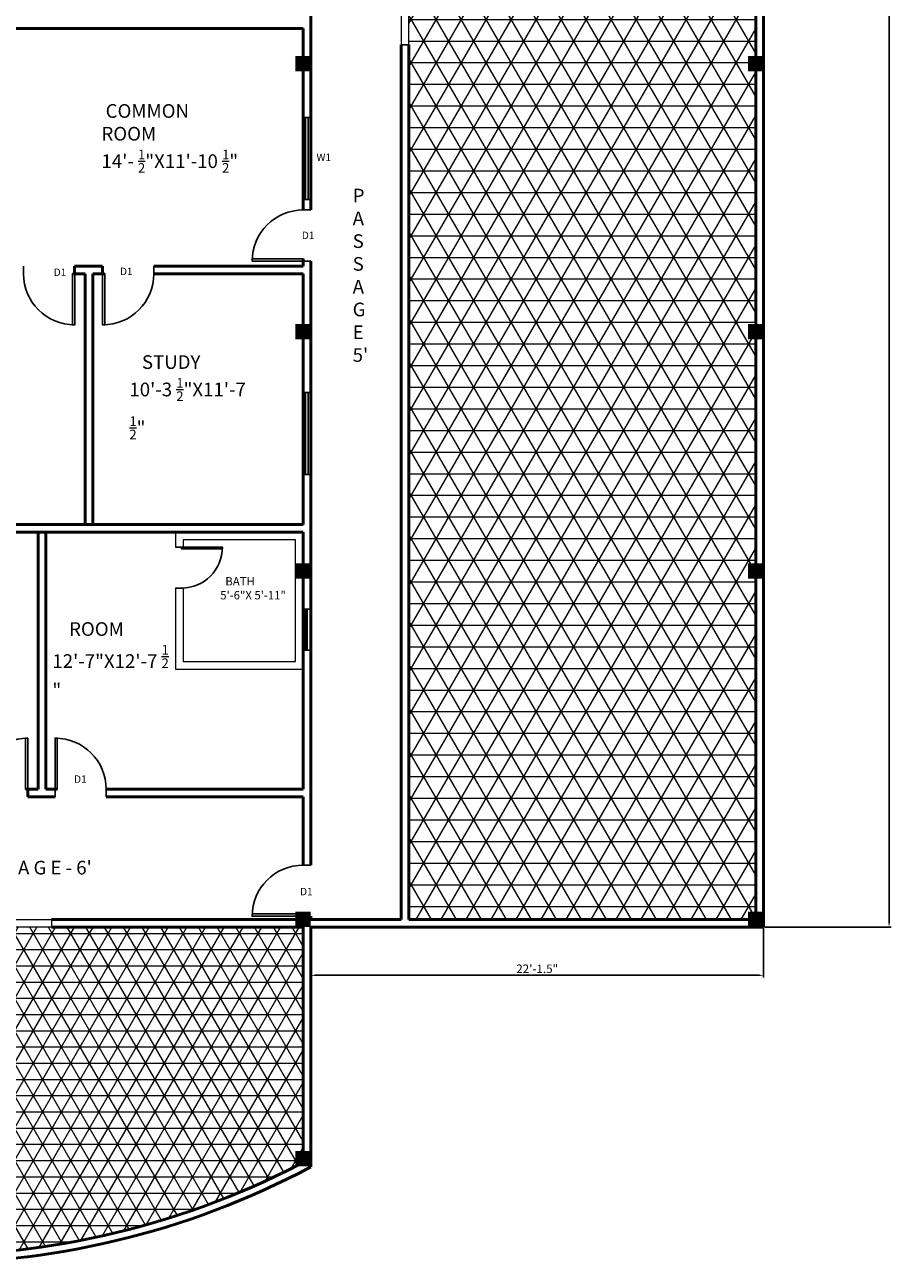
# Model space of a CAD drawing. Units: inches. Extents: x -2733 to 3435, y -338 to 1843.
# Tile 6 of 7: x 1232 to 1741, y 349 to 1076. Entities that reach past the tile are written whole.
import ezdxf

# ---------------------------------------------------------------- set-up
doc = ezdxf.new("R2010")
doc.units = ezdxf.units.IN
doc.header["$PDMODE"] = 34
for name, color, linetype, lineweight in [('A-ANNO-DIMS', 2, 'Continuous', 18), ('A-ANNO-TEXT', 7, 'Continuous', 18), ('A-AREA-IDEN', 3, 'Continuous', 18), ('A-COLS', 1, 'Continuous', 35), ('A-DOOR', 1, 'Continuous', 25), ('A-FLOR-FIXT', 8, 'Continuous', 18), ('A-FLOR-PATT', 9, 'Continuous', 13), ('A-GLAZ', 4, 'Continuous', 25), ('A-WALL', 7, 'Continuous', 50)]:
    doc.layers.add(name, color=color, linetype=linetype, lineweight=lineweight)
doc.styles.get("Standard").update_dxf_attribs({"font": 'arial.ttf'})
doc.styles.add('YQ_DIM', font='SUPEROS.SHX', dxfattribs={"width": 0.8, "bigfont": 'HZDX.SHX'})
doc.dimstyles.new('ISO-25', dxfattribs={"dimtxt": 5, "dimasz": 2.5, "dimexe": 1.25, "dimexo": 0.625, "dimtad": 1, "dimlunit": 3, "dimtxsty": 'Standard', "dimcen": 2.5, "dimadec": 0, "dimazin": 0, "dimtfac": 1, "dimtmove": 0, "dimatfit": 3, "dimfxl": 1, "dimarcsym": 0})

# ---------------------------------------------------------------- blocks, each defined once
blk = doc.blocks.new('*U21')
for p, q in [((0, 0), (0, -6)), ((40, 0), (40, -6))]:
    blk.add_line(p, q)
blk.add_lwpolyline([(0, 0), (0, 40), (1.75, 40), (1.75, 0)], close=True)
blk.add_arc((0, 0), 40, 0, 90)
blk = doc.blocks.new('*D23')
at = {"layer": 'A-ANNO-DIMS', "color": 0, "lineweight": -2, "transparency": 16777216}
for p, q in [((1666.36, 1675.07), (1740.68, 1675.07)), ((1739.43, 1672.57), (1739.43, 549.07)), ((1666.36, 546.57), (1740.68, 546.57))]:
    blk.add_line(p, q, dxfattribs=at)
at = {"layer": 'A-ANNO-DIMS', "color": 0, "lineweight": 20, "transparency": 16777216}
for points in [[(1739.02, 1672.57), (1739.85, 1672.57), (1739.43, 1675.07)], [(1739.02, 549.07), (1739.85, 549.07), (1739.43, 546.57)]]:
    blk.add_solid(points, dxfattribs=at)
at = {"layer": 'Defpoints', "color": 0, "lineweight": 20, "transparency": 16777216}
for p in [(1665.73, 1675.07), (1665.73, 546.57), (1739.43, 546.57)]:
    blk.add_point(p, dxfattribs=at)
at = {"layer": 'A-ANNO-DIMS', "color": 0, "transparency": 16777216, "insert": (1736.26, 1110.82), "char_height": 5, "attachment_point": 5, "rotation": 90}
blk.add_mtext('94\'-0.5"', dxfattribs=at)
blk = doc.blocks.new('*D28')
at = {"layer": 'A-ANNO-DIMS', "color": 0, "lineweight": -2, "ltscale": 0.5, "transparency": 16777216}
for p, q in [((1665.73, 545.95), (1665.73, 517.09)), ((1400.23, 530.41), (1400.23, 517.09)), ((1402.73, 518.34), (1663.23, 518.34))]:
    blk.add_line(p, q, dxfattribs=at)
at = {"layer": 'A-ANNO-DIMS', "color": 0, "lineweight": 20, "ltscale": 0.5, "transparency": 16777216}
for points in [[(1402.73, 518.76), (1402.73, 517.92), (1400.23, 518.34)], [(1663.23, 518.76), (1663.23, 517.92), (1665.73, 518.34)]]:
    blk.add_solid(points, dxfattribs=at)
at = {"layer": 'Defpoints', "color": 0, "lineweight": 20, "ltscale": 0.5, "transparency": 16777216}
for p in [(1665.73, 546.57), (1400.23, 531.04), (1665.73, 518.34)]:
    blk.add_point(p, dxfattribs=at)
at = {"layer": 'A-ANNO-DIMS', "color": 0, "ltscale": 0.5, "transparency": 16777216, "insert": (1532.98, 521.52), "char_height": 5, "attachment_point": 5}
blk.add_mtext('22\'-1.5"', dxfattribs=at)
blk = doc.blocks.new('WIN-1200')
for points in [[(0, 48), (4.5, 48), (4.5, 0), (0, 0)], [(1.29, 48), (2.82, 48), (2.82, 0), (1.29, 0)]]:
    blk.add_lwpolyline(points, close=True)
blk = doc.blocks.new('VENT-600')
at = {"ltscale": 0.5}
for points in [[(0, 24), (4.5, 24), (4.5, 0), (0, 0)], [(1.39, 24), (2.25, 24), (2.25, 0), (1.39, 0)]]:
    blk.add_lwpolyline(points, close=True, dxfattribs=at)

msp = doc.modelspace()

# ---------------------------------------------------------------- hatches: boundary and pattern name
at = {"layer": 'A-COLS'}
h = msp.add_hatch(color=256, dxfattribs=at)
h.dxf.hatch_style = 1
h.paths.add_polyline_path([(1400.159, 1057.953), (1391.159, 1057.953), (1391.159, 1048.953), (1400.159, 1048.953)])
h = msp.add_hatch(color=256, dxfattribs=at)
h.dxf.hatch_style = 1
h.paths.add_polyline_path([(1665.735, 1057.953), (1656.735, 1057.953), (1656.735, 1048.953), (1665.735, 1048.953)])
h = msp.add_hatch(color=256, dxfattribs=at)
h.dxf.hatch_style = 1
h.paths.add_polyline_path([(1400.159, 900.631), (1391.159, 900.631), (1391.159, 891.631), (1400.159, 891.631)])
h = msp.add_hatch(color=256, dxfattribs=at)
h.dxf.hatch_style = 1
h.paths.add_polyline_path([(1665.735, 900.631), (1656.735, 900.631), (1656.735, 891.631), (1665.735, 891.631)])
h = msp.add_hatch(color=256, dxfattribs=at)
h.dxf.hatch_style = 1
h.paths.add_polyline_path([(1400.159, 760.101), (1391.159, 760.101), (1391.159, 751.101), (1400.159, 751.101)])
h = msp.add_hatch(color=256, dxfattribs=at)
h.dxf.hatch_style = 1
h.paths.add_polyline_path([(1665.735, 760.101), (1656.735, 760.101), (1656.735, 751.101), (1665.735, 751.101)])
h = msp.add_hatch(color=256, dxfattribs=at)
h.dxf.hatch_style = 1
h.paths.add_polyline_path([(1400.159, 555.665), (1391.159, 555.665), (1391.159, 546.665), (1400.159, 546.665)])
h = msp.add_hatch(color=256, dxfattribs=at)
h.dxf.hatch_style = 1
h.paths.add_polyline_path([(1665.735, 555.665), (1656.735, 555.665), (1656.735, 546.665), (1665.735, 546.665)])
h = msp.add_hatch(color=256, dxfattribs=at)
h.dxf.hatch_style = 1
h.paths.add_polyline_path([(1400.159, 415.169), (1391.159, 415.169), (1391.159, 406.169), (1400.159, 406.169)])
at = {"layer": 'A-FLOR-PATT'}
h = msp.add_hatch(dxfattribs=at)
h.set_pattern_fill('NET3', color=256, scale=4)
h.paths.add_polyline_path([(1661.235, 1509.072), (1656.735, 1509.072), (1656.735, 1517.29), (1457.735, 1517.29), (1457.735, 1513.572), (1487.735, 1513.572), (1487.735, 1512.26), (1487.706, 1512.26, -0.4014527), (1457.735, 1483.572), (1457.735, 551.072), (1661.235, 551.072)])
h = msp.add_hatch(dxfattribs=at)
h.set_pattern_fill('NET3', color=256, scale=3)
h.paths.add_polyline_path([(1395.735, 546.572), (1089.235, 546.572), (1089.235, 492.572), (964.407, 526.719), (942.472, 413.369, 0.252088), (1395.735, 408.558)])

# ---------------------------------------------------------------- linework, layer by layer
at = {"layer": 'A-FLOR-FIXT', "ltscale": 0.5}
for p, q in [((1453.235, 1214.213), (1453.235, 1064.597)), ((1457.735, 1064.597), (1457.735, 1214.213)), ((1453.235, 1064.597), (1457.735, 1064.597)), ((1176.117, 551.072), (1248.117, 551.072)), ((1248.117, 546.572), (1176.117, 546.572)), ((1248.117, 551.072), (1248.117, 546.572))]:
    msp.add_line(p, q, dxfattribs=at)
at = {"layer": 'A-FLOR-FIXT'}
for p, q in [((1395.735, 967.628), (1400.235, 967.628)), ((1308.059, 934.572), (1308.059, 930.156)), ((1395.735, 937.628), (1400.235, 937.628)), ((1320.735, 769.698), (1325.235, 769.698)), ((1320.735, 745.698), (1325.235, 745.698)), ((1280.124, 627.572), (1280.124, 623.072)), ((1400.235, 583.043), (1395.735, 583.043)), ((1395.735, 553.043), (1400.235, 553.043))]:
    msp.add_line(p, q, dxfattribs=at)
for points in [[(1320.735, 745.698), (1320.735, 698.072), (1395.735, 698.072), (1395.735, 778.572), (1320.735, 778.572), (1320.735, 769.698)], [(1325.235, 745.714), (1325.235, 702.572), (1391.235, 702.572), (1391.235, 774.072), (1325.235, 774.072), (1325.235, 768.648)]]:
    msp.add_lwpolyline(points, dxfattribs=at)
at = {"layer": 'A-GLAZ', "ltscale": 0.5}
msp.add_line((1453.235, 1064.597), (1457.735, 1064.597), dxfattribs=at)
at = {"layer": 'A-WALL'}
for p, q in [((1665.735, 1675.072), (1665.735, 546.572)), ((1661.235, 1509.072), (1661.235, 551.072)), ((1400.235, 1082.676), (1400.235, 967.628)), ((1395.735, 1074.072), (1221.235, 1074.072)), ((1395.735, 1074.072), (1395.735, 967.628)), ((1453.235, 1064.597), (1453.235, 551.072)), ((1457.735, 1064.597), (1457.735, 551.072)), ((1395.735, 938.941), (1395.735, 934.572)), ((1261.606, 934.572), (1261.606, 930.072)), ((1277.992, 934.572), (1261.606, 934.572)), ((1277.992, 934.572), (1277.992, 930.072)), ((1395.735, 934.572), (1308.059, 934.572)), ((1400.235, 937.628), (1400.235, 583.043)), ((1267.735, 930.072), (1260.556, 930.072)), ((1267.735, 930.072), (1267.735, 783.072)), ((1272.235, 930.072), (1272.235, 783.072)), ((1279.042, 930.072), (1272.235, 930.072)), ((1395.735, 930.072), (1308.059, 930.072)), ((1395.735, 930.072), (1395.735, 783.072)), ((1395.735, 783.072), (1018.896, 783.072)), ((1395.735, 778.572), (1089.235, 778.572)), ((1240.235, 778.572), (1240.235, 627.572)), ((1244.735, 778.572), (1244.735, 627.572)), ((1395.735, 778.572), (1395.735, 627.572)), ((1240.235, 627.572), (1233.067, 627.572)), ((1234.117, 627.572), (1234.117, 623.072)), ((1251.437, 627.572), (1244.735, 627.572)), ((1395.735, 627.572), (1280.124, 627.572)), ((1250.124, 623.072), (1234.117, 623.072)), ((1395.735, 623.072), (1280.124, 623.072)), ((1395.735, 623.072), (1395.735, 583.043)), ((1395.735, 554.355), (1395.735, 551.072)), ((1400.235, 553.043), (1400.235, 551.072)), ((1395.735, 551.072), (1248.117, 551.072)), ((1395.735, 546.572), (1248.117, 546.572)), ((1395.735, 546.572), (1395.735, 408.558)), ((1453.235, 551.072), (1400.235, 551.072)), ((1665.735, 546.572), (1400.235, 546.572)), ((1400.235, 546.572), (1400.235, 405.846)), ((1661.235, 551.072), (1457.735, 551.072))]:
    msp.add_line(p, q, dxfattribs=at)
for radius, start, end in [(478.102, 240.087713, 298.300235), (482.602, 240.258112, 298.012953)]:
    msp.add_arc((1173.571, 831.907), radius, start, end, dxfattribs=at)

# ---------------------------------------------------------------- block references
at = {"layer": 'A-DOOR'}
for p, xscale, yscale, zscale, rotation in [((1395.735, 937.628), 0.75, 0.75, 0.75, 90.00000000000003), ((1261.674, 930.156), 0.75, 0.75, 0.75, 180), ((1278.059, 930.156), -0.75, 0.75, 0.75, 180), ((1324.335, 769.698), 0.6, 0.6, 0.6, 270), ((1395.735, 553.043), 0.75, 0.75, 0.75, 90.00000000000003)]:
    msp.add_blockref('*U21', p, dxfattribs=dict(at, xscale=xscale, yscale=yscale, zscale=zscale, rotation=rotation))
at = {"layer": 'A-DOOR', "yscale": 0.75, "zscale": 0.75}
for p, xscale in [((1234.117, 627.572), -0.75), ((1250.124, 627.572), 0.75)]:
    msp.add_blockref('*U21', p, dxfattribs=dict(at, xscale=xscale))
at = {"layer": 'A-GLAZ'}
for name, p in [('WIN-1200', (1395.735, 973.83)), ('WIN-1200', (1395.735, 812.391)), ('VENT-600', (1395.735, 709.242))]:
    msp.add_blockref(name, p, dxfattribs=at)

# ---------------------------------------------------------------- texts
at = {"layer": 'A-ANNO-TEXT', "ltscale": 0.5, "char_height": 4.35068, "attachment_point": 1, "style": 'YQ_DIM'}
for s, insert in [('{\\f@Arial Unicode MS|b0|i0|c0|p34;W1}', (1403.521, 1000.7)), ('{\\f@Arial Unicode MS|b0|i0|c0|p34;D1}', (1394.931, 954.911)), ('{\\f@Arial Unicode MS|b0|i0|c0|p34;D1}', (1249.322, 933.244)), ('{\\f@Arial Unicode MS|b0|i0|c0|p34;D1}', (1288.224, 933.724)), ('{\\f@Arial Unicode MS|b0|i0|c0|p34;D1}', (1261.314, 635.687)), ('{\\f@Arial Unicode MS|b0|i0|c0|p34;D1}', (1393.857, 569.655))]:
    msp.add_mtext_dynamic_manual_height_columns(s, width=7.90712, gutter_width=21.753, heights=[0], dxfattribs=dict(at, insert=insert))
at = {"layer": 'A-AREA-IDEN', "ltscale": 0.5, "attachment_point": 1, "style": 'YQ_DIM'}
for s, width, gutter_width, heights, insert, char_height in [('\\A1;{\\f@Malgun Gothic|b0|i0|c0|p34; COMMON  ROOM \\P14\'- \\H0.7x;\\S1/2;\\H1.42857x;"X11\'-10 \\H0.7x;\\S1/2;\\H1.42857x;"}', 88.00213, 40.122, [0], (1277.356, 1029.762), 8.02448), ("{\\f@Arial Unicode MS|b0|i0|c0|p34;P\\PA\\PS\\PS\\PA\\PG\\PE\\P5'}", 12.11312, 12.5, [123.216], (1424.736, 980.086), 8.02), ('\\A1;{\\f@Malgun Gothic|b0|i0|c0|p34;   STUDY\\P10\'-3 \\H0.7x;\\S1/2;\\H1.42857x;"X11\'-7 \\H0.7x;\\S1/2;\\H1.42857x;"}', 69.89446, 40.122, [0], (1293.744, 882.355), 8.02448), ('\\A1;{  \\fSegoe UI Black|b0|i0|c0|p34;BATH\\P5\'-6\\H1x;"X 5\'-11"}', 43.60909, 24.448, [0], (1347.049, 752.071), 4.88966), ('\\A1;{\\f@Malgun Gothic|b0|i0|c0|p34;    ROOM \\P12\'-7\\H1x;"X12\'-7 \\H0.7x;\\S1/2;\\H1.42857x;"}', 69.89446, 40.122, [0], (1248.558, 725.631), 8.02448)]:
    msp.add_mtext_dynamic_manual_height_columns(s, width=width, gutter_width=gutter_width, heights=heights, dxfattribs=dict(at, insert=insert, char_height=char_height))
at = {"layer": 'A-AREA-IDEN', "insert": (1231.87, 581.536), "char_height": 8, "attachment_point": 5, "style": 'YQ_DIM'}
msp.add_mtext_dynamic_manual_height_columns("{\\f@MS PGothic|b0|i0|c0|p34;P A S S A G E - 6'}", width=111.08232, gutter_width=12.5, heights=[0], dxfattribs=at)

# ---------------------------------------------------------------- dimensions: what is measured, and where the dimension line sits
at = {"layer": 'A-ANNO-DIMS'}
dim = msp.add_linear_dim(base=(1739.434, 546.572), p1=(1665.735, 1675.072), p2=(1665.735, 546.572), angle=90, dimstyle='ISO-25', override={"dimclrd": 0, "dimclre": 0, "dimclrt": 0}, dxfattribs=at)
dim.commit()
dim.dimension.update_dxf_attribs({"geometry": '*D23', "text_midpoint": (1736.256, 1110.822)})
at = {"layer": 'A-ANNO-DIMS', "ltscale": 0.5}
dim = msp.add_linear_dim(base=(1665.735, 518.341), p1=(1400.235, 531.04), p2=(1665.735, 546.572), dimstyle='ISO-25', override={"dimclrd": 0, "dimclre": 0, "dimclrt": 0}, dxfattribs=at)
dim.commit()
dim.dimension.update_dxf_attribs({"geometry": '*D28', "text_midpoint": (1532.985, 521.519)})

doc.saveas('drawing.dxf')
